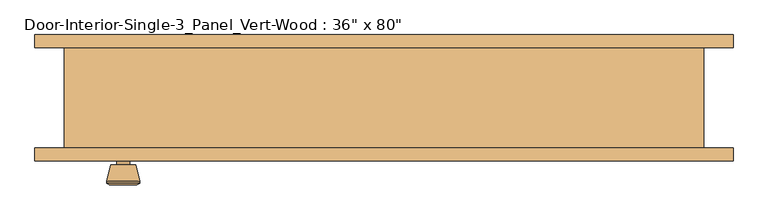
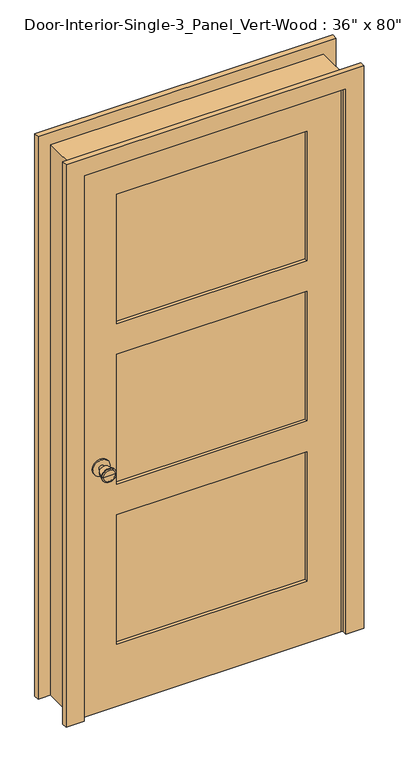
"""IFC4 building model written with IfcOpenShell, lengths in millimetres: door geometry."""

from ifc_helpers import new_model, si_unit, point, frame, frame_2d, origin, place, context, project, spatial, polyline, circle_curve, trimmed, segment, composite_curve, outline, extrude, faceted_brep, source, transform, mapped, element, save
from ifc_brep_helpers import plane_surface, cylinder_surface, revolved_surface, advanced_brep


def door_c5233792(model_context):
    return source(origin(), model_context, "Body", "SolidModel", [
        advanced_brep(
        [(-393.7, -32.1, 914.4), (-403.7, -32.1, 914.4), (-383.7, -32.1, 914.4), (-373.2241324, 16.9, 914.4), (-414.1758676, 16.9, 914.4), (-393.7, 16.9, 914.4), (-368.7, 15.0721319, 914.4), (-418.7, 15.0721319, 914.4), (-368.7, 11.6084537, 914.4), (-418.7, 11.6084537, 914.4), (-375.063764, -13.1, 914.4), (-412.336236, -13.1, 914.4), (-383.7, -13.1, 914.4), (-403.7, -13.1, 914.4)],
        [
            (0, 1),
            (1, 2, circle_curve(frame((-393.7, -32.1, 914.4), z_axis=(0.0, -1.0, 0.0), x_axis=(-1.0, 0.0, 0.0)), 10.0)),
            (2, 0),
            (2, 1, circle_curve(frame((-393.7, -32.1, 914.4), z_axis=(0.0, -1.0, 0.0), x_axis=(-1.0, 0.0, 0.0)), 10.0)),
            (3, 4, circle_curve(frame((-393.7, 16.9, 914.4), z_axis=(0.0, 1.0, 0.0), x_axis=(-1.0, 0.0, 0.0)), 20.4758676)),
            (4, 5),
            (5, 3),
            (4, 3, circle_curve(frame((-393.7, 16.9, 914.4), z_axis=(0.0, 1.0, 0.0), x_axis=(-1.0, 0.0, 0.0)), 20.4758676)),
            (6, 7, circle_curve(frame((-393.7, 15.0721319, 914.4), z_axis=(0.0, 1.0, 0.0), x_axis=(-1.0, 0.0, 0.0)), 25.0)),
            (7, 4),
            (3, 6),
            (7, 6, circle_curve(frame((-393.7, 15.0721319, 914.4), z_axis=(0.0, 1.0, 0.0), x_axis=(-1.0, 0.0, 0.0)), 25.0)),
            (8, 9, circle_curve(frame((-393.7, 11.6084537, 914.4), z_axis=(0.0, 1.0, 0.0), x_axis=(-1.0, 0.0, 0.0)), 25.0)),
            (9, 7),
            (6, 8),
            (9, 8, circle_curve(frame((-393.7, 11.6084537, 914.4), z_axis=(0.0, 1.0, 0.0), x_axis=(-1.0, 0.0, 0.0)), 25.0)),
            (10, 11, circle_curve(frame((-393.7, -13.1, 914.4), z_axis=(0.0, 1.0, 0.0), x_axis=(-1.0, 0.0, 0.0)), 18.636236)),
            (11, 9),
            (8, 10),
            (11, 10, circle_curve(frame((-393.7, -13.1, 914.4), z_axis=(0.0, 1.0, 0.0), x_axis=(-1.0, 0.0, 0.0)), 18.636236)),
            (12, 13, circle_curve(frame((-393.7, -13.1, 914.4), z_axis=(0.0, 1.0, 0.0), x_axis=(-1.0, 0.0, 0.0)), 10.0)),
            (13, 11),
            (10, 12),
            (13, 12, circle_curve(frame((-393.7, -13.1, 914.4), z_axis=(0.0, 1.0, 0.0), x_axis=(-1.0, 0.0, 0.0)), 10.0)),
            (1, 13),
            (12, 2),
        ],
        [
            plane_surface(frame((-393.7, -32.1, 914.4), z_axis=(0.0, -1.0, 0.0), x_axis=(-1.0, 0.0, 0.0))),
            plane_surface(frame((-393.7, 16.9, 914.4), z_axis=(0.0, 1.0, 0.0), x_axis=(-1.0, 0.0, 0.0))),
            revolved_surface(polyline([(-414.1758676, 16.9, 914.4), (-418.7, 15.0721319, 914.4)]), (-393.7, -32.1, 914.4), (0.0, -1.0, 0.0)),
            cylinder_surface(frame((-393.7, -32.1, 914.4), z_axis=(0.0, -1.0, 0.0), x_axis=(-1.0, 0.0, 0.0)), 25.0),
            revolved_surface(polyline([(-418.7, 11.6084537, 914.4), (-412.336236, -13.1, 914.4)]), (-393.7, -32.1, 914.4), (0.0, -1.0, 0.0)),
            plane_surface(frame((-393.7, -13.1, 914.4), z_axis=(0.0, -1.0, 0.0), x_axis=(-1.0, 0.0, 0.0))),
            cylinder_surface(frame((-393.7, -32.1, 914.4), z_axis=(0.0, -1.0, 0.0), x_axis=(-1.0, 0.0, 0.0)), 10.0),
        ],
        [
            (0, [[1, 2, 3]]),
            (0, [[-3, 4, -1]]),
            (1, [[5, 6, 7]]),
            (1, [[8, -7, -6]]),
            (2, [[9, 10, -5, 11]]),
            (2, [[12, -11, -8, -10]]),
            (3, [[13, 14, -9, 15]]),
            (3, [[16, -15, -12, -14]]),
            (4, [[17, 18, -13, 19]]),
            (4, [[20, -19, -16, -18]]),
            (5, [[21, 22, -17, 23]]),
            (5, [[24, -23, -20, -22]]),
            (6, [[-2, 25, -21, 26]]),
            (6, [[-4, -26, -24, -25]]),
        ],
    ),
        extrude(outline(composite_curve([segment(trimmed(circle_curve(frame_2d((914.4, -393.7)), 30.0), [point((914.4, -423.7))], [point((914.4, -363.7))], False, "CARTESIAN"), True, "CONTINUOUS"), segment(trimmed(circle_curve(frame_2d((914.4, -393.7)), 30.0), [point((914.4, -363.7))], [point((914.4, -423.7))], False, "CARTESIAN"), True, "CONTINUOUS")], self_intersect=False)), frame((0.0, -38.1, 0.0), z_axis=(0.0, 1.0, 0.0), x_axis=(0.0, 0.0, 1.0)), (0.0, 0.0, 1.0), 6.0),
        advanced_brep(
        [(-393.7, -79.025, 914.4), (-383.7, -79.025, 914.4), (-403.7, -79.025, 914.4), (-373.2241324, -128.025, 914.4), (-393.7, -128.025, 914.4), (-414.1758676, -128.025, 914.4), (-368.7, -126.1971319, 914.4), (-418.7, -126.1971319, 914.4), (-368.7, -122.7334537, 914.4), (-418.7, -122.7334537, 914.4), (-375.063764, -98.025, 914.4), (-412.336236, -98.025, 914.4), (-383.7, -98.025, 914.4), (-403.7, -98.025, 914.4)],
        [
            (0, 1),
            (1, 2, circle_curve(frame((-393.7, -79.025, 914.4), z_axis=(0.0, 1.0, 0.0), x_axis=(-1.0, 0.0, 0.0)), 10.0)),
            (2, 0),
            (2, 1, circle_curve(frame((-393.7, -79.025, 914.4), z_axis=(0.0, 1.0, 0.0), x_axis=(-1.0, 0.0, 0.0)), 10.0)),
            (3, 4),
            (4, 5),
            (5, 3, circle_curve(frame((-393.7, -128.025, 914.4), z_axis=(0.0, -1.0, 0.0), x_axis=(-1.0, 0.0, 0.0)), 20.4758676)),
            (3, 5, circle_curve(frame((-393.7, -128.025, 914.4), z_axis=(0.0, -1.0, 0.0), x_axis=(-1.0, 0.0, 0.0)), 20.4758676)),
            (6, 3),
            (5, 7),
            (7, 6, circle_curve(frame((-393.7, -126.1971319, 914.4), z_axis=(0.0, -1.0, 0.0), x_axis=(-1.0, 0.0, 0.0)), 25.0)),
            (6, 7, circle_curve(frame((-393.7, -126.1971319, 914.4), z_axis=(0.0, -1.0, 0.0), x_axis=(-1.0, 0.0, 0.0)), 25.0)),
            (8, 6),
            (7, 9),
            (9, 8, circle_curve(frame((-393.7, -122.7334537, 914.4), z_axis=(0.0, -1.0, 0.0), x_axis=(-1.0, 0.0, 0.0)), 25.0)),
            (8, 9, circle_curve(frame((-393.7, -122.7334537, 914.4), z_axis=(0.0, -1.0, 0.0), x_axis=(-1.0, 0.0, 0.0)), 25.0)),
            (10, 8),
            (9, 11),
            (11, 10, circle_curve(frame((-393.7, -98.025, 914.4), z_axis=(0.0, -1.0, 0.0), x_axis=(-1.0, 0.0, 0.0)), 18.636236)),
            (10, 11, circle_curve(frame((-393.7, -98.025, 914.4), z_axis=(0.0, -1.0, 0.0), x_axis=(-1.0, 0.0, 0.0)), 18.636236)),
            (12, 10),
            (11, 13),
            (13, 12, circle_curve(frame((-393.7, -98.025, 914.4), z_axis=(0.0, -1.0, 0.0), x_axis=(-1.0, 0.0, 0.0)), 10.0)),
            (12, 13, circle_curve(frame((-393.7, -98.025, 914.4), z_axis=(0.0, -1.0, 0.0), x_axis=(-1.0, 0.0, 0.0)), 10.0)),
            (1, 12),
            (13, 2),
        ],
        [
            plane_surface(frame((-393.7, -79.025, 914.4), z_axis=(0.0, 1.0, 0.0), x_axis=(-1.0, 0.0, 0.0))),
            plane_surface(frame((-393.7, -128.025, 914.4), z_axis=(0.0, -1.0, 0.0), x_axis=(-1.0, 0.0, 0.0))),
            revolved_surface(polyline([(-414.1758676, -128.025, 914.4), (-418.7, -126.1971319, 914.4)]), (-393.7, -79.025, 914.4), (0.0, 1.0, 0.0)),
            cylinder_surface(frame((-393.7, -79.025, 914.4), z_axis=(0.0, 1.0, 0.0), x_axis=(-1.0, 0.0, 0.0)), 25.0),
            revolved_surface(polyline([(-418.7, -122.7334537, 914.4), (-412.336236, -98.025, 914.4)]), (-393.7, -79.025, 914.4), (0.0, 1.0, 0.0)),
            plane_surface(frame((-393.7, -98.025, 914.4), z_axis=(0.0, 1.0, 0.0), x_axis=(-1.0, 0.0, 0.0))),
            cylinder_surface(frame((-393.7, -79.025, 914.4), z_axis=(0.0, 1.0, 0.0), x_axis=(-1.0, 0.0, 0.0)), 10.0),
        ],
        [
            (0, [[1, 2, 3]]),
            (0, [[-3, 4, -1]]),
            (1, [[5, 6, 7]]),
            (1, [[-6, -5, 8]]),
            (2, [[9, -7, 10, 11]]),
            (2, [[-10, -8, -9, 12]]),
            (3, [[13, -11, 14, 15]]),
            (3, [[-14, -12, -13, 16]]),
            (4, [[17, -15, 18, 19]]),
            (4, [[-18, -16, -17, 20]]),
            (5, [[21, -19, 22, 23]]),
            (5, [[-22, -20, -21, 24]]),
            (6, [[25, -23, 26, -2]]),
            (6, [[-26, -24, -25, -4]]),
        ],
    ),
        extrude(outline(composite_curve([segment(trimmed(circle_curve(frame_2d((914.4, -393.7)), 30.0), [point((914.4, -423.7))], [point((914.4, -363.7))], False, "CARTESIAN"), True, "CONTINUOUS"), segment(trimmed(circle_curve(frame_2d((914.4, -393.7)), 30.0), [point((914.4, -363.7))], [point((914.4, -423.7))], False, "CARTESIAN"), True, "CONTINUOUS")], self_intersect=False)), frame((0.0, -79.025, 0.0), z_axis=(0.0, 1.0, 0.0), x_axis=(0.0, 0.0, 1.0)), (0.0, 0.0, 1.0), 6.0),
        extrude(outline(polyline([(336.55, -49.7416667), (336.55, -61.3833333), (-336.55, -61.3833333), (-336.55, -49.7416667), (336.55, -49.7416667)])), frame((0.0, 0.0, 1428.75), z_axis=(0.0, 0.0, 1.0), x_axis=(1.0, 0.0, 0.0)), (0.0, 0.0, 1.0), 484.1875),
        extrude(outline(polyline([(336.55, -49.7416667), (336.55, -61.3833333), (-336.55, -61.3833333), (-336.55, -49.7416667), (336.55, -49.7416667)])), frame((0.0, 0.0, 231.775), z_axis=(0.0, 0.0, 1.0), x_axis=(1.0, 0.0, 0.0)), (0.0, 0.0, 1.0), 484.1875),
        extrude(outline(polyline([(336.55, -49.7416667), (336.55, -61.3833333), (-336.55, -61.3833333), (-336.55, -49.7416667), (336.55, -49.7416667)])), frame((0.0, 0.0, 830.2625), z_axis=(0.0, 0.0, 1.0), x_axis=(1.0, 0.0, 0.0)), (0.0, 0.0, 1.0), 484.1875),
        extrude(outline(polyline([(2032.0, -457.2), (0.0, -457.2), (0.0, 457.2), (2032.0, 457.2), (2032.0, -457.2)]), holes=[polyline([(1912.9375, -336.55), (1912.9375, 336.55), (1428.75, 336.55), (1428.75, -336.55), (1912.9375, -336.55)]), polyline([(715.9625, -336.55), (715.9625, 336.55), (231.775, 336.55), (231.775, -336.55), (715.9625, -336.55)]), polyline([(1314.45, -336.55), (1314.45, 336.55), (830.2625, 336.55), (830.2625, -336.55), (1314.45, -336.55)])]), frame((0.0, -73.025, 0.0), z_axis=(0.0, 1.0, 0.0), x_axis=(0.0, 0.0, 1.0)), (0.0, 0.0, 1.0), 34.925),
        faceted_brep([(482.6, -73.025, 0.0), (457.2, -73.025, 0.0), (457.2, -38.1, 0.0), (444.5, -38.1, 0.0), (444.5, -3.175, 0.0), (457.2, -3.175, 0.0), (457.2, 79.375, 0.0), (482.6, 79.375, 0.0), (482.6, 79.375, 2057.4), (482.6, -73.025, 2057.4), (457.2, 79.375, 2032.0), (-457.2, 79.375, 2032.0), (-457.2, 79.375, 0.0), (-482.6, 79.375, 0.0), (-482.6, 79.375, 2057.4), (457.2, -3.175, 2032.0), (444.5, -3.175, 2019.3), (-444.5, -3.175, 2019.3), (-444.5, -3.175, 0.0), (-457.2, -3.175, 0.0), (-457.2, -3.175, 2032.0), (444.5, -38.1, 2019.3), (457.2, -38.1, 2032.0), (-457.2, -38.1, 2032.0), (-457.2, -38.1, 0.0), (-444.5, -38.1, 0.0), (-444.5, -38.1, 2019.3), (457.2, -73.025, 2032.0), (-482.6, -73.025, 2057.4), (-482.6, -73.025, 0.0), (-457.2, -73.025, 0.0), (-457.2, -73.025, 2032.0)], [[[0, 1, 2, 3, 4, 5, 6, 7]], [[7, 8, 9, 0]], [[6, 10, 11, 12, 13, 14, 8, 7]], [[5, 15, 10, 6]], [[4, 16, 17, 18, 19, 20, 15, 5]], [[3, 21, 16, 4]], [[2, 22, 23, 24, 25, 26, 21, 3]], [[1, 27, 22, 2]], [[0, 9, 28, 29, 30, 31, 27, 1]], [[8, 14, 28, 9]], [[15, 20, 11, 10]], [[21, 26, 17, 16]], [[27, 31, 23, 22]], [[29, 13, 12, 19, 18, 25, 24, 30]], [[14, 13, 29, 28]], [[20, 19, 12, 11]], [[26, 25, 18, 17]], [[31, 30, 24, 23]]]),
        extrude(outline(polyline([(0.0, 527.05), (2101.85, 527.05), (2101.85, -527.05), (0.0, -527.05), (0.0, -463.55), (2038.35, -463.55), (2038.35, 463.55), (0.0, 463.55), (0.0, 527.05)])), frame((0.0, 79.375, 0.0), z_axis=(0.0, 1.0, 0.0), x_axis=(0.0, 0.0, 1.0)), (0.0, 0.0, 1.0), 19.05),
        extrude(outline(polyline([(0.0, 527.05), (2101.85, 527.05), (2101.85, -527.05), (0.0, -527.05), (0.0, -463.55), (2038.35, -463.55), (2038.35, 463.55), (0.0, 463.55), (0.0, 527.05)])), frame((0.0, -92.075, 0.0), z_axis=(0.0, 1.0, 0.0), x_axis=(0.0, 0.0, 1.0)), (0.0, 0.0, 1.0), 19.05),
    ])


if __name__ == "__main__":
    model = new_model("IFC4")
    model_context = context("Model", 3, world=origin())
    ifc_project = project(units=[si_unit("LENGTHUNIT", "METRE", prefix="MILLI")], contexts=[model_context])
    site = spatial("IfcSite", under=ifc_project)
    building = spatial("IfcBuilding", under=site)
    placement = place(None, origin())
    door_shape = door_c5233792(model_context)
    element("IfcDoor", 1, ObjectType="Door-Interior-Single-3_Panel_Vert-Wood : 36\" x 80\"", at=placement, inside=building, context=model_context, shape_type="MappedRepresentation", body=[
        mapped(door_shape, transform((0.0, 0.0, 0.0), x_axis=(1.0, 0.0, 0.0), y_axis=(0.0, 1.0, 0.0), z_axis=(0.0, 0.0, 1.0))),
    ])
    save(model, "model.ifc")

# Revit data of these elements
# Type "Door-Interior-Single-3_Panel_Vert-Wood : 36\" x 80\""
#   Type Mark = "10"
#   Assembly Code = "C1020300"
#   Analytic Construction = "Wooden"
#   Top Rail = 0' - 4 11/16"
#   Thickness = 0' - 1 3/8"
#   Thermal Resistance (R) = 2.5876 (h·ft²·°F)/BTU
#   Swing Angle [instance default] = 90.00°
#   Stiles = 0' - 4 3/4"
#   Rough Width = 3' - 2"
#   Rough Height = 6' - 9"
#   Intermediate Rail = 0' - 4 1/2"
#   Height = 6' - 8"
#   Width = 3' - 0"
#   Heat Transfer Coefficient (U) = 0.3865 BTU/(h·ft²·°F)
#   Bottom Rail = 0' - 9 1/8"
#   Trim Material = Cherry
#   Panel Material = Cherry
#   Frame Material = Cherry
#   Door Handle Material = Aluminum
#   Visual Light Transmittance = 0
#   Solar Heat Gain Coefficient = 0
#   Wall Closure = (empty or 0)
#   Function = (empty or 0)
# Element 1 (IfcDoor, "Door-Interior-Single-3_Panel_Vert-Wood : 36\" x 80\"")
#   Materials on its faces: "Cherry", "Aluminum"
# Materials
#   "Cherry": class "Wood", colour RGB 226 177 128, transparency 0, Description = "Prunus Serotina", Cost = 0
#   "Aluminum": class "Metal", colour RGB 247 247 247, transparency 0, Description = "Aluminum 6061", Cost = 0
